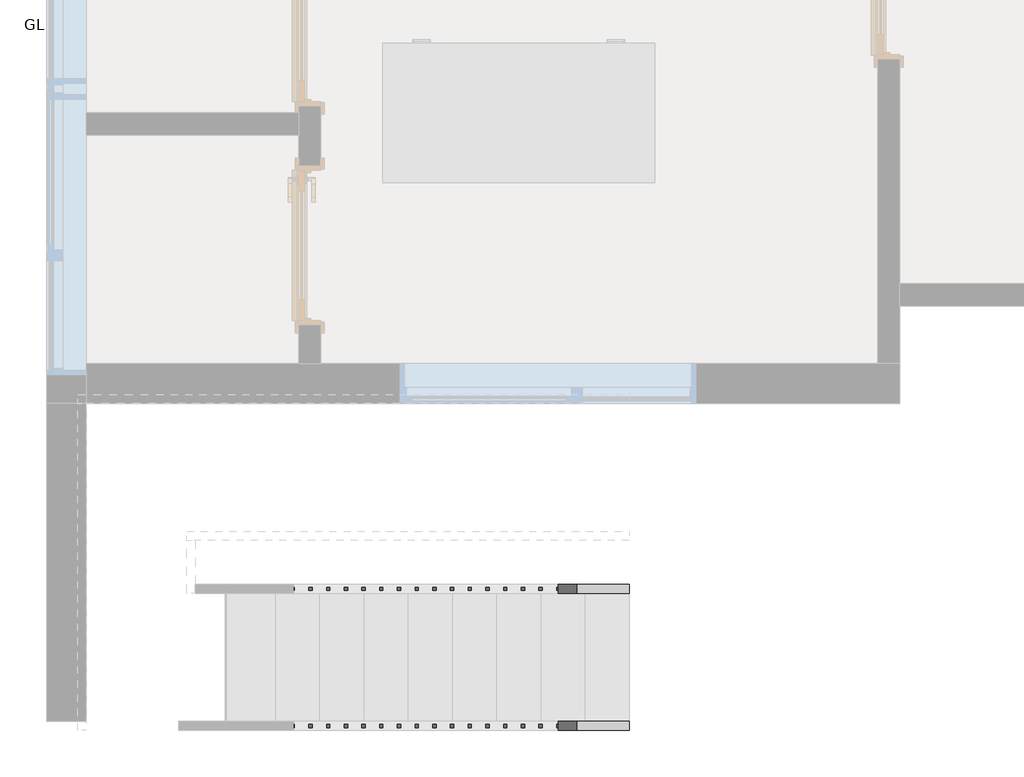
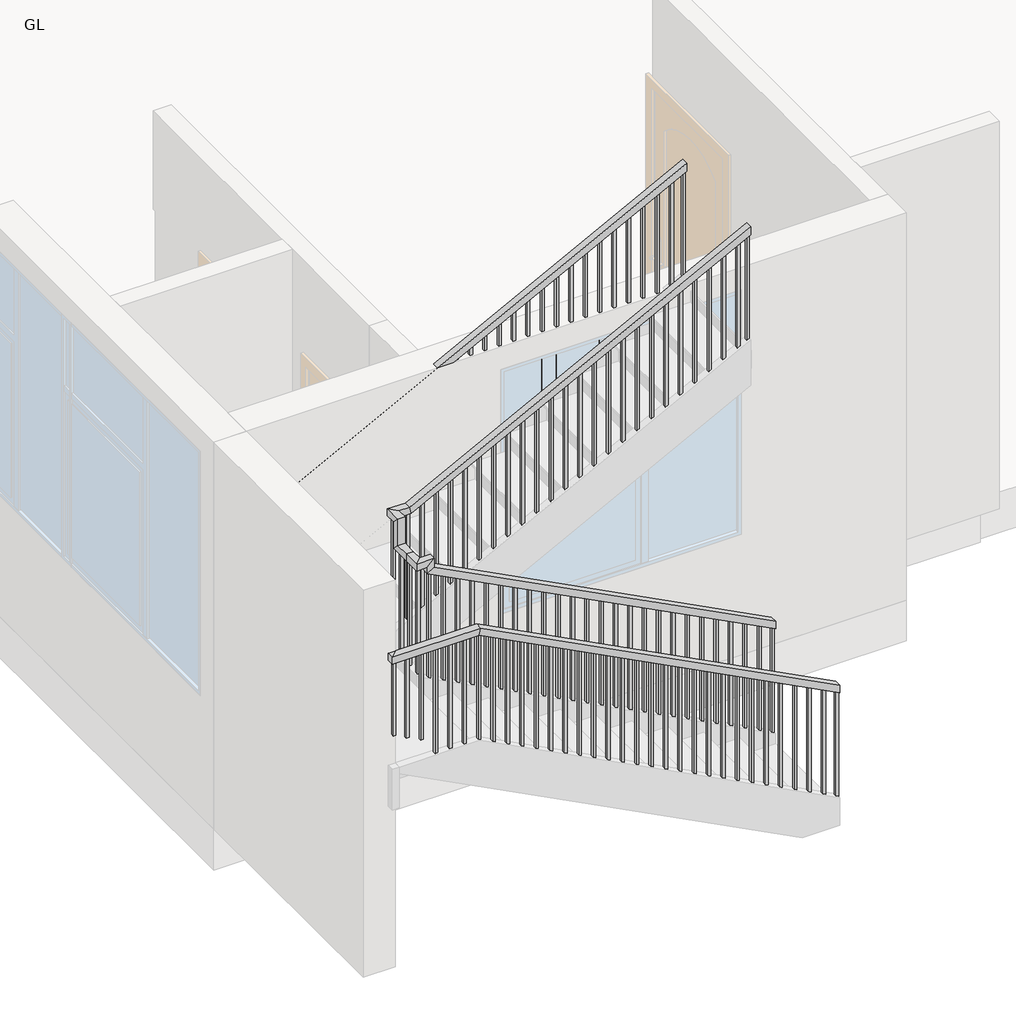
# One storey, part 3 of 4: 2 railings.
"""IFC4 building model written with IfcOpenShell, lengths in millimetres."""

from ifc_helpers import new_model, si_unit, frame, origin, place, context, project, spatial, polyline, outline, extrude, faceted_brep, element, save

model = new_model("IFC4")

# Units and contexts
model_context = context("Model", 3, world=origin())
ifc_project = project(units=[si_unit("LENGTHUNIT", "METRE", prefix="MILLI")], contexts=[model_context])

# Site, building, storey
site = spatial("IfcSite", under=ifc_project)
building = spatial("IfcBuilding", under=site)
storey = spatial("IfcBuildingStorey", under=building, Name="GL", Elevation=0.0)

# Railings
placement = place(None, origin())
element("IfcRailing", 1, ObjectType="Handrail - Rectangular", at=placement, inside=storey, context=model_context, shape_type="SolidModel", body=[
    faceted_brep([(-3117.2664982, -6914.3822004, 1046.0181818), (-3117.2664982, -6914.3822004, 988.803028), (-3117.2664982, -6863.5822004, 988.803028), (-3117.2664982, -6863.5822004, 1046.0181818), (-5530.2664982, -6914.3822004, 2296.3909091), (-5581.0664982, -6914.3822004, 2265.4993916), (-5581.0664982, -6863.5822004, 2265.4993916), (-5530.2664982, -6863.5822004, 2296.3909091), (-5657.2664982, -6787.3822004, 2311.4), (-5657.2664982, -6787.3822004, 2362.2), (-5657.2664982, -6685.7822004, 2362.2), (-5657.2664982, -6634.9822004, 2311.4), (-5606.4664982, -6787.3822004, 2311.4), (-5606.4664982, -6634.9822004, 2311.4), (-5606.4664982, -6787.3822004, 2362.2), (-5606.4664982, -6685.7822004, 2362.2), (-3117.2664982, -6558.7822004, 3810.0), (-3117.2664982, -6609.5822004, 3810.0), (-3117.2664982, -6609.5822004, 3752.7848461), (-3117.2664982, -6558.7822004, 3752.7848461), (-5517.8863767, -6558.7822004, 2508.8272727), (-5530.2664982, -6558.7822004, 2559.6272727), (-5517.8863767, -6609.5822004, 2508.8272727), (-5530.2664982, -6609.5822004, 2559.6272727), (-5530.2664982, -6914.3822004, 2362.2), (-5581.0664982, -6914.3822004, 2311.4), (-5581.0664982, -6863.5822004, 2311.4), (-5530.2664982, -6863.5822004, 2362.2), (-5657.2664982, -6914.3822004, 2362.2), (-5657.2664982, -6914.3822004, 2311.4), (-5606.4664982, -6863.5822004, 2311.4), (-5606.4664982, -6863.5822004, 2362.2), (-5657.2664982, -6685.7822004, 2559.6272727), (-5657.2664982, -6634.9822004, 2508.8272727), (-5606.4664982, -6634.9822004, 2508.8272727), (-5606.4664982, -6685.7822004, 2559.6272727), (-5657.2664982, -6558.7822004, 2559.6272727), (-5657.2664982, -6558.7822004, 2508.8272727), (-5606.4664982, -6609.5822004, 2508.8272727), (-5606.4664982, -6609.5822004, 2559.6272727)], [[[0, 1, 2, 3]], [[1, 0, 4, 5]], [[2, 1, 5, 6]], [[3, 2, 6, 7]], [[0, 3, 7, 4]], [[8, 9, 10, 11]], [[12, 8, 11, 13]], [[14, 12, 13, 15]], [[9, 14, 15, 10]], [[16, 17, 18, 19]], [[20, 21, 16, 19]], [[22, 20, 19, 18]], [[23, 22, 18, 17]], [[21, 23, 17, 16]], [[5, 4, 24, 25]], [[6, 5, 25, 26]], [[7, 6, 26, 27]], [[4, 7, 27, 24]], [[25, 24, 28, 29]], [[26, 25, 29, 30]], [[27, 26, 30, 31]], [[24, 27, 31, 28]], [[29, 28, 9, 8]], [[30, 29, 8, 12]], [[31, 30, 12, 14]], [[28, 31, 14, 9]], [[11, 10, 32, 33]], [[13, 11, 33, 34]], [[15, 13, 34, 35]], [[10, 15, 35, 32]], [[33, 32, 36, 37]], [[34, 33, 37, 38]], [[35, 34, 38, 39]], [[32, 35, 39, 36]], [[37, 36, 21, 20]], [[38, 37, 20, 22]], [[39, 38, 22, 23]], [[36, 39, 23, 21]]]),
    extrude(outline(polyline([(3718.2350734, -3183.9414982), (3708.3637098, -3202.9914982), (2924.0803899, -3202.9914982), (2933.9517536, -3183.9414982), (3718.2350734, -3183.9414982)])), frame((0.0, -6593.7072004, 0.0), z_axis=(0.0, 1.0, 0.0), x_axis=(0.0, 0.0, 1.0)), (0.0, 0.0, 1.0), 19.05),
    extrude(outline(polyline([(3665.5878007, -3285.5414982), (3655.716437, -3304.5914982), (2871.4331172, -3304.5914982), (2881.3044808, -3285.5414982), (3665.5878007, -3285.5414982)])), frame((0.0, -6593.7072004, 0.0), z_axis=(0.0, 1.0, 0.0), x_axis=(0.0, 0.0, 1.0)), (0.0, 0.0, 1.0), 19.05),
    extrude(outline(polyline([(3612.940528, -3387.1414982), (3603.0691643, -3406.1914982), (2818.7858445, -3406.1914982), (2828.6572081, -3387.1414982), (3612.940528, -3387.1414982)])), frame((0.0, -6593.7072004, 0.0), z_axis=(0.0, 1.0, 0.0), x_axis=(0.0, 0.0, 1.0)), (0.0, 0.0, 1.0), 19.05),
    extrude(outline(polyline([(3560.2932552, -3488.7414982), (3550.4218916, -3507.7914982), (2766.1385718, -3507.7914982), (2776.0099354, -3488.7414982), (3560.2932552, -3488.7414982)])), frame((0.0, -6593.7072004, 0.0), z_axis=(0.0, 1.0, 0.0), x_axis=(0.0, 0.0, 1.0)), (0.0, 0.0, 1.0), 19.05),
    extrude(outline(polyline([(3507.6459825, -3590.3414982), (3497.7746189, -3609.3914982), (2713.491299, -3609.3914982), (2723.3626627, -3590.3414982), (3507.6459825, -3590.3414982)])), frame((0.0, -6593.7072004, 0.0), z_axis=(0.0, 1.0, 0.0), x_axis=(0.0, 0.0, 1.0)), (0.0, 0.0, 1.0), 19.05),
    extrude(outline(polyline([(3454.9987098, -3691.9414982), (3445.1273461, -3710.9914982), (2660.8440263, -3710.9914982), (2670.7153899, -3691.9414982), (3454.9987098, -3691.9414982)])), frame((0.0, -6593.7072004, 0.0), z_axis=(0.0, 1.0, 0.0), x_axis=(0.0, 0.0, 1.0)), (0.0, 0.0, 1.0), 19.05),
    extrude(outline(polyline([(3402.351437, -3793.5414982), (3392.4800734, -3812.5914982), (2608.1967536, -3812.5914982), (2618.0681172, -3793.5414982), (3402.351437, -3793.5414982)])), frame((0.0, -6593.7072004, 0.0), z_axis=(0.0, 1.0, 0.0), x_axis=(0.0, 0.0, 1.0)), (0.0, 0.0, 1.0), 19.05),
    extrude(outline(polyline([(3349.7041643, -3895.1414982), (3339.8328007, -3914.1914982), (2555.5494808, -3914.1914982), (2565.4208445, -3895.1414982), (3349.7041643, -3895.1414982)])), frame((0.0, -6593.7072004, 0.0), z_axis=(0.0, 1.0, 0.0), x_axis=(0.0, 0.0, 1.0)), (0.0, 0.0, 1.0), 19.05),
    extrude(outline(polyline([(3297.0568916, -3996.7414982), (3287.185528, -4015.7914982), (2502.9022081, -4015.7914982), (2512.7735718, -3996.7414982), (3297.0568916, -3996.7414982)])), frame((0.0, -6593.7072004, 0.0), z_axis=(0.0, 1.0, 0.0), x_axis=(0.0, 0.0, 1.0)), (0.0, 0.0, 1.0), 19.05),
    extrude(outline(polyline([(3244.4096189, -4098.3414982), (3234.5382552, -4117.3914982), (2450.2549354, -4117.3914982), (2460.126299, -4098.3414982), (3244.4096189, -4098.3414982)])), frame((0.0, -6593.7072004, 0.0), z_axis=(0.0, 1.0, 0.0), x_axis=(0.0, 0.0, 1.0)), (0.0, 0.0, 1.0), 19.05),
    extrude(outline(polyline([(3191.7623461, -4199.9414982), (3181.8909825, -4218.9914982), (2397.6076627, -4218.9914982), (2407.4790263, -4199.9414982), (3191.7623461, -4199.9414982)])), frame((0.0, -6593.7072004, 0.0), z_axis=(0.0, 1.0, 0.0), x_axis=(0.0, 0.0, 1.0)), (0.0, 0.0, 1.0), 19.05),
    extrude(outline(polyline([(3139.1150734, -4301.5414982), (3129.2437098, -4320.5914982), (2344.9603899, -4320.5914982), (2354.8317536, -4301.5414982), (3139.1150734, -4301.5414982)])), frame((0.0, -6593.7072004, 0.0), z_axis=(0.0, 1.0, 0.0), x_axis=(0.0, 0.0, 1.0)), (0.0, 0.0, 1.0), 19.05),
    extrude(outline(polyline([(3086.4678007, -4403.1414982), (3076.596437, -4422.1914982), (2292.3131172, -4422.1914982), (2302.1844808, -4403.1414982), (3086.4678007, -4403.1414982)])), frame((0.0, -6593.7072004, 0.0), z_axis=(0.0, 1.0, 0.0), x_axis=(0.0, 0.0, 1.0)), (0.0, 0.0, 1.0), 19.05),
    extrude(outline(polyline([(3033.820528, -4504.7414982), (3023.9491643, -4523.7914982), (2239.6658445, -4523.7914982), (2249.5372081, -4504.7414982), (3033.820528, -4504.7414982)])), frame((0.0, -6593.7072004, 0.0), z_axis=(0.0, 1.0, 0.0), x_axis=(0.0, 0.0, 1.0)), (0.0, 0.0, 1.0), 19.05),
    extrude(outline(polyline([(2981.1732552, -4606.3414982), (2971.3018916, -4625.3914982), (2187.0185718, -4625.3914982), (2196.8899354, -4606.3414982), (2981.1732552, -4606.3414982)])), frame((0.0, -6593.7072004, 0.0), z_axis=(0.0, 1.0, 0.0), x_axis=(0.0, 0.0, 1.0)), (0.0, 0.0, 1.0), 19.05),
    extrude(outline(polyline([(2928.5259825, -4707.9414982), (2918.6546189, -4726.9914982), (2134.371299, -4726.9914982), (2144.2426627, -4707.9414982), (2928.5259825, -4707.9414982)])), frame((0.0, -6593.7072004, 0.0), z_axis=(0.0, 1.0, 0.0), x_axis=(0.0, 0.0, 1.0)), (0.0, 0.0, 1.0), 19.05),
    extrude(outline(polyline([(2875.8787098, -4809.5414982), (2866.0073461, -4828.5914982), (2081.7240263, -4828.5914982), (2091.5953899, -4809.5414982), (2875.8787098, -4809.5414982)])), frame((0.0, -6593.7072004, 0.0), z_axis=(0.0, 1.0, 0.0), x_axis=(0.0, 0.0, 1.0)), (0.0, 0.0, 1.0), 19.05),
    extrude(outline(polyline([(2823.231437, -4911.1414982), (2813.3600734, -4930.1914982), (2029.0767536, -4930.1914982), (2038.9481172, -4911.1414982), (2823.231437, -4911.1414982)])), frame((0.0, -6593.7072004, 0.0), z_axis=(0.0, 1.0, 0.0), x_axis=(0.0, 0.0, 1.0)), (0.0, 0.0, 1.0), 19.05),
    extrude(outline(polyline([(2770.5841643, -5012.7414982), (2760.7128007, -5031.7914982), (1976.4294808, -5031.7914982), (1986.3008445, -5012.7414982), (2770.5841643, -5012.7414982)])), frame((0.0, -6593.7072004, 0.0), z_axis=(0.0, 1.0, 0.0), x_axis=(0.0, 0.0, 1.0)), (0.0, 0.0, 1.0), 19.05),
    extrude(outline(polyline([(2717.9368916, -5114.3414982), (2708.065528, -5133.3914982), (1923.7822081, -5133.3914982), (1933.6535718, -5114.3414982), (2717.9368916, -5114.3414982)])), frame((0.0, -6593.7072004, 0.0), z_axis=(0.0, 1.0, 0.0), x_axis=(0.0, 0.0, 1.0)), (0.0, 0.0, 1.0), 19.05),
    extrude(outline(polyline([(2665.2896189, -5215.9414982), (2655.4182552, -5234.9914982), (1871.1349354, -5234.9914982), (1881.006299, -5215.9414982), (2665.2896189, -5215.9414982)])), frame((0.0, -6593.7072004, 0.0), z_axis=(0.0, 1.0, 0.0), x_axis=(0.0, 0.0, 1.0)), (0.0, 0.0, 1.0), 19.05),
    extrude(outline(polyline([(2612.6423461, -5317.5414982), (2602.7709825, -5336.5914982), (1818.4876627, -5336.5914982), (1828.3590263, -5317.5414982), (2612.6423461, -5317.5414982)])), frame((0.0, -6593.7072004, 0.0), z_axis=(0.0, 1.0, 0.0), x_axis=(0.0, 0.0, 1.0)), (0.0, 0.0, 1.0), 19.05),
    extrude(outline(polyline([(2559.9950734, -5419.1414982), (2550.1237098, -5438.1914982), (1765.8403899, -5438.1914982), (1775.7117536, -5419.1414982), (2559.9950734, -5419.1414982)])), frame((0.0, -6593.7072004, 0.0), z_axis=(0.0, 1.0, 0.0), x_axis=(0.0, 0.0, 1.0)), (0.0, 0.0, 1.0), 19.05),
    extrude(outline(polyline([(2507.3478007, -5520.7414982), (2497.476437, -5539.7914982), (1713.1931172, -5539.7914982), (1723.0644808, -5520.7414982), (2507.3478007, -5520.7414982)])), frame((0.0, -6593.7072004, 0.0), z_axis=(0.0, 1.0, 0.0), x_axis=(0.0, 0.0, 1.0)), (0.0, 0.0, 1.0), 19.05),
    extrude(outline(polyline([(-5622.3414982, -6695.3072004), (-5641.3914982, -6695.3072004), (-5641.3914982, -6676.2572004), (-5622.3414982, -6676.2572004), (-5622.3414982, -6695.3072004)])), frame((0.0, 0.0, 1524.0), z_axis=(0.0, 0.0, 1.0), x_axis=(1.0, 0.0, 0.0)), (0.0, 0.0, 1.0), 787.4),
    extrude(outline(polyline([(-5622.3414982, -6796.9072004), (-5641.3914982, -6796.9072004), (-5641.3914982, -6777.8572004), (-5622.3414982, -6777.8572004), (-5622.3414982, -6796.9072004)])), frame((0.0, 0.0, 1524.0), z_axis=(0.0, 0.0, 1.0), x_axis=(1.0, 0.0, 0.0)), (0.0, 0.0, 1.0), 787.4),
    extrude(outline(polyline([(2311.4, -5546.1414982), (2311.4, -5565.1914982), (1472.9899354, -5565.1914982), (1463.1185718, -5546.1414982), (2311.4, -5546.1414982)])), frame((0.0, -6898.5072004, 0.0), z_axis=(0.0, 1.0, 0.0), x_axis=(0.0, 0.0, 1.0)), (0.0, 0.0, 1.0), 19.05),
    extrude(outline(polyline([(2194.7546189, -5444.5414982), (2204.6259825, -5463.5914982), (1420.3426627, -5463.5914982), (1410.471299, -5444.5414982), (2194.7546189, -5444.5414982)])), frame((0.0, -6898.5072004, 0.0), z_axis=(0.0, 1.0, 0.0), x_axis=(0.0, 0.0, 1.0)), (0.0, 0.0, 1.0), 19.05),
    extrude(outline(polyline([(2142.1073461, -5342.9414982), (2151.9787098, -5361.9914982), (1367.6953899, -5361.9914982), (1357.8240263, -5342.9414982), (2142.1073461, -5342.9414982)])), frame((0.0, -6898.5072004, 0.0), z_axis=(0.0, 1.0, 0.0), x_axis=(0.0, 0.0, 1.0)), (0.0, 0.0, 1.0), 19.05),
    extrude(outline(polyline([(2089.4600734, -5241.3414982), (2099.331437, -5260.3914982), (1315.0481172, -5260.3914982), (1305.1767536, -5241.3414982), (2089.4600734, -5241.3414982)])), frame((0.0, -6898.5072004, 0.0), z_axis=(0.0, 1.0, 0.0), x_axis=(0.0, 0.0, 1.0)), (0.0, 0.0, 1.0), 19.05),
    extrude(outline(polyline([(2036.8128007, -5139.7414982), (2046.6841643, -5158.7914982), (1262.4008445, -5158.7914982), (1252.5294808, -5139.7414982), (2036.8128007, -5139.7414982)])), frame((0.0, -6898.5072004, 0.0), z_axis=(0.0, 1.0, 0.0), x_axis=(0.0, 0.0, 1.0)), (0.0, 0.0, 1.0), 19.05),
    extrude(outline(polyline([(1984.165528, -5038.1414982), (1994.0368916, -5057.1914982), (1209.7535718, -5057.1914982), (1199.8822081, -5038.1414982), (1984.165528, -5038.1414982)])), frame((0.0, -6898.5072004, 0.0), z_axis=(0.0, 1.0, 0.0), x_axis=(0.0, 0.0, 1.0)), (0.0, 0.0, 1.0), 19.05),
    extrude(outline(polyline([(1931.5182552, -4936.5414982), (1941.3896189, -4955.5914982), (1157.106299, -4955.5914982), (1147.2349354, -4936.5414982), (1931.5182552, -4936.5414982)])), frame((0.0, -6898.5072004, 0.0), z_axis=(0.0, 1.0, 0.0), x_axis=(0.0, 0.0, 1.0)), (0.0, 0.0, 1.0), 19.05),
    extrude(outline(polyline([(1878.8709825, -4834.9414982), (1888.7423461, -4853.9914982), (1104.4590263, -4853.9914982), (1094.5876627, -4834.9414982), (1878.8709825, -4834.9414982)])), frame((0.0, -6898.5072004, 0.0), z_axis=(0.0, 1.0, 0.0), x_axis=(0.0, 0.0, 1.0)), (0.0, 0.0, 1.0), 19.05),
    extrude(outline(polyline([(1826.2237098, -4733.3414982), (1836.0950734, -4752.3914982), (1051.8117536, -4752.3914982), (1041.9403899, -4733.3414982), (1826.2237098, -4733.3414982)])), frame((0.0, -6898.5072004, 0.0), z_axis=(0.0, 1.0, 0.0), x_axis=(0.0, 0.0, 1.0)), (0.0, 0.0, 1.0), 19.05),
    extrude(outline(polyline([(1773.576437, -4631.7414982), (1783.4478007, -4650.7914982), (999.1644808, -4650.7914982), (989.2931172, -4631.7414982), (1773.576437, -4631.7414982)])), frame((0.0, -6898.5072004, 0.0), z_axis=(0.0, 1.0, 0.0), x_axis=(0.0, 0.0, 1.0)), (0.0, 0.0, 1.0), 19.05),
    extrude(outline(polyline([(1720.9291643, -4530.1414982), (1730.800528, -4549.1914982), (946.5172081, -4549.1914982), (936.6458445, -4530.1414982), (1720.9291643, -4530.1414982)])), frame((0.0, -6898.5072004, 0.0), z_axis=(0.0, 1.0, 0.0), x_axis=(0.0, 0.0, 1.0)), (0.0, 0.0, 1.0), 19.05),
    extrude(outline(polyline([(1668.2818916, -4428.5414982), (1678.1532552, -4447.5914982), (893.8699354, -4447.5914982), (883.9985718, -4428.5414982), (1668.2818916, -4428.5414982)])), frame((0.0, -6898.5072004, 0.0), z_axis=(0.0, 1.0, 0.0), x_axis=(0.0, 0.0, 1.0)), (0.0, 0.0, 1.0), 19.05),
    extrude(outline(polyline([(1615.6346189, -4326.9414982), (1625.5059825, -4345.9914982), (841.2226627, -4345.9914982), (831.351299, -4326.9414982), (1615.6346189, -4326.9414982)])), frame((0.0, -6898.5072004, 0.0), z_axis=(0.0, 1.0, 0.0), x_axis=(0.0, 0.0, 1.0)), (0.0, 0.0, 1.0), 19.05),
    extrude(outline(polyline([(1562.9873461, -4225.3414982), (1572.8587098, -4244.3914982), (788.5753899, -4244.3914982), (778.7040263, -4225.3414982), (1562.9873461, -4225.3414982)])), frame((0.0, -6898.5072004, 0.0), z_axis=(0.0, 1.0, 0.0), x_axis=(0.0, 0.0, 1.0)), (0.0, 0.0, 1.0), 19.05),
    extrude(outline(polyline([(1510.3400734, -4123.7414982), (1520.211437, -4142.7914982), (735.9281172, -4142.7914982), (726.0567536, -4123.7414982), (1510.3400734, -4123.7414982)])), frame((0.0, -6898.5072004, 0.0), z_axis=(0.0, 1.0, 0.0), x_axis=(0.0, 0.0, 1.0)), (0.0, 0.0, 1.0), 19.05),
    extrude(outline(polyline([(1457.6928007, -4022.1414982), (1467.5641643, -4041.1914982), (683.2808445, -4041.1914982), (673.4094808, -4022.1414982), (1457.6928007, -4022.1414982)])), frame((0.0, -6898.5072004, 0.0), z_axis=(0.0, 1.0, 0.0), x_axis=(0.0, 0.0, 1.0)), (0.0, 0.0, 1.0), 19.05),
    extrude(outline(polyline([(1405.045528, -3920.5414982), (1414.9168916, -3939.5914982), (630.6335718, -3939.5914982), (620.7622081, -3920.5414982), (1405.045528, -3920.5414982)])), frame((0.0, -6898.5072004, 0.0), z_axis=(0.0, 1.0, 0.0), x_axis=(0.0, 0.0, 1.0)), (0.0, 0.0, 1.0), 19.05),
    extrude(outline(polyline([(1352.3982552, -3818.9414982), (1362.2696189, -3837.9914982), (577.986299, -3837.9914982), (568.1149354, -3818.9414982), (1352.3982552, -3818.9414982)])), frame((0.0, -6898.5072004, 0.0), z_axis=(0.0, 1.0, 0.0), x_axis=(0.0, 0.0, 1.0)), (0.0, 0.0, 1.0), 19.05),
    extrude(outline(polyline([(1299.7509825, -3717.3414982), (1309.6223461, -3736.3914982), (525.3390263, -3736.3914982), (515.4676627, -3717.3414982), (1299.7509825, -3717.3414982)])), frame((0.0, -6898.5072004, 0.0), z_axis=(0.0, 1.0, 0.0), x_axis=(0.0, 0.0, 1.0)), (0.0, 0.0, 1.0), 19.05),
    extrude(outline(polyline([(1247.1037098, -3615.7414982), (1256.9750734, -3634.7914982), (472.6917536, -3634.7914982), (462.8203899, -3615.7414982), (1247.1037098, -3615.7414982)])), frame((0.0, -6898.5072004, 0.0), z_axis=(0.0, 1.0, 0.0), x_axis=(0.0, 0.0, 1.0)), (0.0, 0.0, 1.0), 19.05),
    extrude(outline(polyline([(1194.456437, -3514.1414982), (1204.3278007, -3533.1914982), (420.0444808, -3533.1914982), (410.1731172, -3514.1414982), (1194.456437, -3514.1414982)])), frame((0.0, -6898.5072004, 0.0), z_axis=(0.0, 1.0, 0.0), x_axis=(0.0, 0.0, 1.0)), (0.0, 0.0, 1.0), 19.05),
    extrude(outline(polyline([(1141.8091643, -3412.5414982), (1151.680528, -3431.5914982), (367.3972081, -3431.5914982), (357.5258445, -3412.5414982), (1141.8091643, -3412.5414982)])), frame((0.0, -6898.5072004, 0.0), z_axis=(0.0, 1.0, 0.0), x_axis=(0.0, 0.0, 1.0)), (0.0, 0.0, 1.0), 19.05),
    extrude(outline(polyline([(1089.1618916, -3310.9414982), (1099.0332552, -3329.9914982), (314.7499354, -3329.9914982), (304.8785718, -3310.9414982), (1089.1618916, -3310.9414982)])), frame((0.0, -6898.5072004, 0.0), z_axis=(0.0, 1.0, 0.0), x_axis=(0.0, 0.0, 1.0)), (0.0, 0.0, 1.0), 19.05),
    extrude(outline(polyline([(1036.5146189, -3209.3414982), (1046.3859825, -3228.3914982), (262.1026627, -3228.3914982), (252.231299, -3209.3414982), (1036.5146189, -3209.3414982)])), frame((0.0, -6898.5072004, 0.0), z_axis=(0.0, 1.0, 0.0), x_axis=(0.0, 0.0, 1.0)), (0.0, 0.0, 1.0), 19.05),
    extrude(outline(polyline([(-6593.7072004, 2508.8272727), (-6574.6572004, 2508.8272727), (-6574.6572004, 1670.4172081), (-6593.7072004, 1660.5458445), (-6593.7072004, 2508.8272727)])), frame((-5641.3914982, 0.0, 0.0), z_axis=(1.0, 0.0, 0.0), x_axis=(0.0, 1.0, 0.0)), (0.0, 0.0, 1.0), 19.05),
    extrude(outline(polyline([(-5622.3414982, -6879.4572004), (-5622.3414982, -6898.5072004), (-5641.3914982, -6898.5072004), (-5641.3914982, -6879.4572004), (-5622.3414982, -6879.4572004)])), frame((0.0, 0.0, 1524.0), z_axis=(0.0, 0.0, 1.0), x_axis=(1.0, 0.0, 0.0)), (0.0, 0.0, 1.0), 787.4),
    extrude(outline(polyline([(3752.7848461, -3117.2664982), (3742.9134825, -3136.3164982), (2958.6301627, -3136.3164982), (2968.5015263, -3117.2664982), (3752.7848461, -3117.2664982)])), frame((0.0, -6593.7072004, 0.0), z_axis=(0.0, 1.0, 0.0), x_axis=(0.0, 0.0, 1.0)), (0.0, 0.0, 1.0), 19.05),
    extrude(outline(polyline([(988.803028, -3117.2664982), (998.6743916, -3136.3164982), (214.3910718, -3136.3164982), (204.5197081, -3117.2664982), (988.803028, -3117.2664982)])), frame((0.0, -6898.5072004, 0.0), z_axis=(0.0, 1.0, 0.0), x_axis=(0.0, 0.0, 1.0)), (0.0, 0.0, 1.0), 19.05),
])
element("IfcRailing", 2, ObjectType="Handrail - Rectangular", at=placement, inside=storey, context=model_context, shape_type="SolidModel", body=[
    faceted_brep([(-3117.2664982, -7701.7822004, 1046.0181818), (-3117.2664982, -7701.7822004, 988.803028), (-3117.2664982, -7650.9822004, 988.803028), (-3117.2664982, -7650.9822004, 1046.0181818), (-5657.2664982, -7701.7822004, 2362.2), (-5669.6466197, -7701.7822004, 2311.4), (-5669.6466197, -7650.9822004, 2311.4), (-5657.2664982, -7650.9822004, 2362.2), (-6283.3131972, -7701.7822004, 2311.4), (-6283.3131972, -7701.7822004, 2362.2), (-6283.3131972, -5773.9082131, 2362.2), (-6283.3131972, -5773.9082131, 2311.4), (-6232.5131972, -7650.9822004, 2311.4), (-6232.5131972, -5824.7082131, 2311.4), (-6232.5131972, -7650.9822004, 2362.2), (-6232.5131972, -5824.7082131, 2362.2), (-5911.2664982, -5773.9082131, 2362.2), (-5898.8863767, -5773.9082131, 2311.4), (-5898.8863767, -5824.7082131, 2311.4), (-5911.2664982, -5824.7082131, 2362.2), (-3117.2664982, -5773.9082131, 3810.0), (-3117.2664982, -5824.7082131, 3810.0), (-3117.2664982, -5824.7082131, 3752.7848461), (-3117.2664982, -5773.9082131, 3752.7848461)], [[[0, 1, 2, 3]], [[1, 0, 4, 5]], [[2, 1, 5, 6]], [[3, 2, 6, 7]], [[0, 3, 7, 4]], [[8, 9, 10, 11]], [[12, 8, 11, 13]], [[14, 12, 13, 15]], [[9, 14, 15, 10]], [[11, 10, 16, 17]], [[13, 11, 17, 18]], [[15, 13, 18, 19]], [[10, 15, 19, 16]], [[5, 4, 9, 8]], [[6, 5, 8, 12]], [[7, 6, 12, 14]], [[4, 7, 14, 9]], [[20, 21, 22, 23]], [[17, 16, 20, 23]], [[18, 17, 23, 22]], [[19, 18, 22, 21]], [[16, 19, 21, 20]]]),
    extrude(outline(polyline([(3699.8413294, -3219.4381972), (2915.5580095, -3219.4381972), (2925.4293732, -3200.3881972), (3709.712693, -3200.3881972), (3699.8413294, -3219.4381972)])), frame((0.0, -5808.8332131, 0.0), z_axis=(0.0, 1.0, 0.0), x_axis=(0.0, 0.0, 1.0)), (0.0, 0.0, 1.0), 19.05),
    extrude(outline(polyline([(3647.1940566, -3321.0381972), (2862.9107368, -3321.0381972), (2872.7821004, -3301.9881972), (3657.0654203, -3301.9881972), (3647.1940566, -3321.0381972)])), frame((0.0, -5808.8332131, 0.0), z_axis=(0.0, 1.0, 0.0), x_axis=(0.0, 0.0, 1.0)), (0.0, 0.0, 1.0), 19.05),
    extrude(outline(polyline([(3594.5467839, -3422.6381972), (2810.2634641, -3422.6381972), (2820.1348277, -3403.5881972), (3604.4181476, -3403.5881972), (3594.5467839, -3422.6381972)])), frame((0.0, -5808.8332131, 0.0), z_axis=(0.0, 1.0, 0.0), x_axis=(0.0, 0.0, 1.0)), (0.0, 0.0, 1.0), 19.05),
    extrude(outline(polyline([(3541.8995112, -3524.2381972), (2757.6161913, -3524.2381972), (2767.487555, -3505.1881972), (3551.7708748, -3505.1881972), (3541.8995112, -3524.2381972)])), frame((0.0, -5808.8332131, 0.0), z_axis=(0.0, 1.0, 0.0), x_axis=(0.0, 0.0, 1.0)), (0.0, 0.0, 1.0), 19.05),
    extrude(outline(polyline([(3489.2522385, -3625.8381972), (2704.9689186, -3625.8381972), (2714.8402823, -3606.7881972), (3499.1236021, -3606.7881972), (3489.2522385, -3625.8381972)])), frame((0.0, -5808.8332131, 0.0), z_axis=(0.0, 1.0, 0.0), x_axis=(0.0, 0.0, 1.0)), (0.0, 0.0, 1.0), 19.05),
    extrude(outline(polyline([(3436.6049657, -3727.4381972), (2652.3216459, -3727.4381972), (2662.1930095, -3708.3881972), (3446.4763294, -3708.3881972), (3436.6049657, -3727.4381972)])), frame((0.0, -5808.8332131, 0.0), z_axis=(0.0, 1.0, 0.0), x_axis=(0.0, 0.0, 1.0)), (0.0, 0.0, 1.0), 19.05),
    extrude(outline(polyline([(3383.957693, -3829.0381972), (2599.6743732, -3829.0381972), (2609.5457368, -3809.9881972), (3393.8290566, -3809.9881972), (3383.957693, -3829.0381972)])), frame((0.0, -5808.8332131, 0.0), z_axis=(0.0, 1.0, 0.0), x_axis=(0.0, 0.0, 1.0)), (0.0, 0.0, 1.0), 19.05),
    extrude(outline(polyline([(3331.3104203, -3930.6381972), (2547.0271004, -3930.6381972), (2556.8984641, -3911.5881972), (3341.1817839, -3911.5881972), (3331.3104203, -3930.6381972)])), frame((0.0, -5808.8332131, 0.0), z_axis=(0.0, 1.0, 0.0), x_axis=(0.0, 0.0, 1.0)), (0.0, 0.0, 1.0), 19.05),
    extrude(outline(polyline([(3278.6631476, -4032.2381972), (2494.3798277, -4032.2381972), (2504.2511913, -4013.1881972), (3288.5345112, -4013.1881972), (3278.6631476, -4032.2381972)])), frame((0.0, -5808.8332131, 0.0), z_axis=(0.0, 1.0, 0.0), x_axis=(0.0, 0.0, 1.0)), (0.0, 0.0, 1.0), 19.05),
    extrude(outline(polyline([(3226.0158748, -4133.8381972), (2441.732555, -4133.8381972), (2451.6039186, -4114.7881972), (3235.8872385, -4114.7881972), (3226.0158748, -4133.8381972)])), frame((0.0, -5808.8332131, 0.0), z_axis=(0.0, 1.0, 0.0), x_axis=(0.0, 0.0, 1.0)), (0.0, 0.0, 1.0), 19.05),
    extrude(outline(polyline([(3173.3686021, -4235.4381972), (2389.0852823, -4235.4381972), (2398.9566459, -4216.3881972), (3183.2399657, -4216.3881972), (3173.3686021, -4235.4381972)])), frame((0.0, -5808.8332131, 0.0), z_axis=(0.0, 1.0, 0.0), x_axis=(0.0, 0.0, 1.0)), (0.0, 0.0, 1.0), 19.05),
    extrude(outline(polyline([(3120.7213294, -4337.0381972), (2336.4380095, -4337.0381972), (2346.3093732, -4317.9881972), (3130.592693, -4317.9881972), (3120.7213294, -4337.0381972)])), frame((0.0, -5808.8332131, 0.0), z_axis=(0.0, 1.0, 0.0), x_axis=(0.0, 0.0, 1.0)), (0.0, 0.0, 1.0), 19.05),
    extrude(outline(polyline([(3068.0740566, -4438.6381972), (2283.7907368, -4438.6381972), (2293.6621004, -4419.5881972), (3077.9454203, -4419.5881972), (3068.0740566, -4438.6381972)])), frame((0.0, -5808.8332131, 0.0), z_axis=(0.0, 1.0, 0.0), x_axis=(0.0, 0.0, 1.0)), (0.0, 0.0, 1.0), 19.05),
    extrude(outline(polyline([(3015.4267839, -4540.2381972), (2231.1434641, -4540.2381972), (2241.0148277, -4521.1881972), (3025.2981476, -4521.1881972), (3015.4267839, -4540.2381972)])), frame((0.0, -5808.8332131, 0.0), z_axis=(0.0, 1.0, 0.0), x_axis=(0.0, 0.0, 1.0)), (0.0, 0.0, 1.0), 19.05),
    extrude(outline(polyline([(2962.7795112, -4641.8381972), (2178.4961913, -4641.8381972), (2188.367555, -4622.7881972), (2972.6508748, -4622.7881972), (2962.7795112, -4641.8381972)])), frame((0.0, -5808.8332131, 0.0), z_axis=(0.0, 1.0, 0.0), x_axis=(0.0, 0.0, 1.0)), (0.0, 0.0, 1.0), 19.05),
    extrude(outline(polyline([(2910.1322385, -4743.4381972), (2125.8489186, -4743.4381972), (2135.7202823, -4724.3881972), (2920.0036021, -4724.3881972), (2910.1322385, -4743.4381972)])), frame((0.0, -5808.8332131, 0.0), z_axis=(0.0, 1.0, 0.0), x_axis=(0.0, 0.0, 1.0)), (0.0, 0.0, 1.0), 19.05),
    extrude(outline(polyline([(2857.4849657, -4845.0381972), (2073.2016459, -4845.0381972), (2083.0730095, -4825.9881972), (2867.3563294, -4825.9881972), (2857.4849657, -4845.0381972)])), frame((0.0, -5808.8332131, 0.0), z_axis=(0.0, 1.0, 0.0), x_axis=(0.0, 0.0, 1.0)), (0.0, 0.0, 1.0), 19.05),
    extrude(outline(polyline([(2804.837693, -4946.6381972), (2020.5543732, -4946.6381972), (2030.4257368, -4927.5881972), (2814.7090566, -4927.5881972), (2804.837693, -4946.6381972)])), frame((0.0, -5808.8332131, 0.0), z_axis=(0.0, 1.0, 0.0), x_axis=(0.0, 0.0, 1.0)), (0.0, 0.0, 1.0), 19.05),
    extrude(outline(polyline([(2752.1904203, -5048.2381972), (1967.9071004, -5048.2381972), (1977.7784641, -5029.1881972), (2762.0617839, -5029.1881972), (2752.1904203, -5048.2381972)])), frame((0.0, -5808.8332131, 0.0), z_axis=(0.0, 1.0, 0.0), x_axis=(0.0, 0.0, 1.0)), (0.0, 0.0, 1.0), 19.05),
    extrude(outline(polyline([(2699.5431476, -5149.8381972), (1915.2598277, -5149.8381972), (1925.1311913, -5130.7881972), (2709.4145112, -5130.7881972), (2699.5431476, -5149.8381972)])), frame((0.0, -5808.8332131, 0.0), z_axis=(0.0, 1.0, 0.0), x_axis=(0.0, 0.0, 1.0)), (0.0, 0.0, 1.0), 19.05),
    extrude(outline(polyline([(2646.8958748, -5251.4381972), (1862.612555, -5251.4381972), (1872.4839186, -5232.3881972), (2656.7672385, -5232.3881972), (2646.8958748, -5251.4381972)])), frame((0.0, -5808.8332131, 0.0), z_axis=(0.0, 1.0, 0.0), x_axis=(0.0, 0.0, 1.0)), (0.0, 0.0, 1.0), 19.05),
    extrude(outline(polyline([(2594.2486021, -5353.0381972), (1809.9652823, -5353.0381972), (1819.8366459, -5333.9881972), (2604.1199657, -5333.9881972), (2594.2486021, -5353.0381972)])), frame((0.0, -5808.8332131, 0.0), z_axis=(0.0, 1.0, 0.0), x_axis=(0.0, 0.0, 1.0)), (0.0, 0.0, 1.0), 19.05),
    extrude(outline(polyline([(2541.6013294, -5454.6381972), (1757.3180095, -5454.6381972), (1767.1893732, -5435.5881972), (2551.472693, -5435.5881972), (2541.6013294, -5454.6381972)])), frame((0.0, -5808.8332131, 0.0), z_axis=(0.0, 1.0, 0.0), x_axis=(0.0, 0.0, 1.0)), (0.0, 0.0, 1.0), 19.05),
    extrude(outline(polyline([(2488.9540566, -5556.2381972), (1704.6707368, -5556.2381972), (1714.5421004, -5537.1881972), (2498.8254203, -5537.1881972), (2488.9540566, -5556.2381972)])), frame((0.0, -5808.8332131, 0.0), z_axis=(0.0, 1.0, 0.0), x_axis=(0.0, 0.0, 1.0)), (0.0, 0.0, 1.0), 19.05),
    extrude(outline(polyline([(2436.3067839, -5657.8381972), (1652.0234641, -5657.8381972), (1661.8948277, -5638.7881972), (2446.1781476, -5638.7881972), (2436.3067839, -5657.8381972)])), frame((0.0, -5808.8332131, 0.0), z_axis=(0.0, 1.0, 0.0), x_axis=(0.0, 0.0, 1.0)), (0.0, 0.0, 1.0), 19.05),
    extrude(outline(polyline([(2383.6595112, -5759.4381972), (1599.3761913, -5759.4381972), (1609.247555, -5740.3881972), (2393.5308748, -5740.3881972), (2383.6595112, -5759.4381972)])), frame((0.0, -5808.8332131, 0.0), z_axis=(0.0, 1.0, 0.0), x_axis=(0.0, 0.0, 1.0)), (0.0, 0.0, 1.0), 19.05),
    extrude(outline(polyline([(2331.0122385, -5861.0381972), (1546.7289186, -5861.0381972), (1556.6002823, -5841.9881972), (2340.8836021, -5841.9881972), (2331.0122385, -5861.0381972)])), frame((0.0, -5808.8332131, 0.0), z_axis=(0.0, 1.0, 0.0), x_axis=(0.0, 0.0, 1.0)), (0.0, 0.0, 1.0), 19.05),
    extrude(outline(polyline([(2311.4, -5962.6381972), (1494.0816459, -5962.6381972), (1503.9530095, -5943.5881972), (2311.4, -5943.5881972), (2311.4, -5962.6381972)])), frame((0.0, -5808.8332131, 0.0), z_axis=(0.0, 1.0, 0.0), x_axis=(0.0, 0.0, 1.0)), (0.0, 0.0, 1.0), 19.05),
    extrude(outline(polyline([(2311.4, -6064.2381972), (1441.4343732, -6064.2381972), (1451.3057368, -6045.1881972), (2311.4, -6045.1881972), (2311.4, -6064.2381972)])), frame((0.0, -5808.8332131, 0.0), z_axis=(0.0, 1.0, 0.0), x_axis=(0.0, 0.0, 1.0)), (0.0, 0.0, 1.0), 19.05),
    extrude(outline(polyline([(2311.4, -6165.8381972), (1388.7871004, -6165.8381972), (1398.6584641, -6146.7881972), (2311.4, -6146.7881972), (2311.4, -6165.8381972)])), frame((0.0, -5808.8332131, 0.0), z_axis=(0.0, 1.0, 0.0), x_axis=(0.0, 0.0, 1.0)), (0.0, 0.0, 1.0), 19.05),
    extrude(outline(polyline([(-6267.4381972, -5857.1072004), (-6267.4381972, -5838.0572004), (-6248.3881972, -5838.0572004), (-6248.3881972, -5857.1072004), (-6267.4381972, -5857.1072004)])), frame((0.0, 0.0, 1524.0), z_axis=(0.0, 0.0, 1.0), x_axis=(1.0, 0.0, 0.0)), (0.0, 0.0, 1.0), 787.4),
    extrude(outline(polyline([(-6267.4381972, -5958.7072004), (-6267.4381972, -5939.6572004), (-6248.3881972, -5939.6572004), (-6248.3881972, -5958.7072004), (-6267.4381972, -5958.7072004)])), frame((0.0, 0.0, 1524.0), z_axis=(0.0, 0.0, 1.0), x_axis=(1.0, 0.0, 0.0)), (0.0, 0.0, 1.0), 787.4),
    extrude(outline(polyline([(-6267.4381972, -6060.3072004), (-6267.4381972, -6041.2572004), (-6248.3881972, -6041.2572004), (-6248.3881972, -6060.3072004), (-6267.4381972, -6060.3072004)])), frame((0.0, 0.0, 1524.0), z_axis=(0.0, 0.0, 1.0), x_axis=(1.0, 0.0, 0.0)), (0.0, 0.0, 1.0), 787.4),
    extrude(outline(polyline([(-6267.4381972, -6161.9072004), (-6267.4381972, -6142.8572004), (-6248.3881972, -6142.8572004), (-6248.3881972, -6161.9072004), (-6267.4381972, -6161.9072004)])), frame((0.0, 0.0, 1524.0), z_axis=(0.0, 0.0, 1.0), x_axis=(1.0, 0.0, 0.0)), (0.0, 0.0, 1.0), 787.4),
    extrude(outline(polyline([(-6267.4381972, -6263.5072004), (-6267.4381972, -6244.4572004), (-6248.3881972, -6244.4572004), (-6248.3881972, -6263.5072004), (-6267.4381972, -6263.5072004)])), frame((0.0, 0.0, 1524.0), z_axis=(0.0, 0.0, 1.0), x_axis=(1.0, 0.0, 0.0)), (0.0, 0.0, 1.0), 787.4),
    extrude(outline(polyline([(-6267.4381972, -6365.1072004), (-6267.4381972, -6346.0572004), (-6248.3881972, -6346.0572004), (-6248.3881972, -6365.1072004), (-6267.4381972, -6365.1072004)])), frame((0.0, 0.0, 1524.0), z_axis=(0.0, 0.0, 1.0), x_axis=(1.0, 0.0, 0.0)), (0.0, 0.0, 1.0), 787.4),
    extrude(outline(polyline([(-6267.4381972, -6466.7072004), (-6267.4381972, -6447.6572004), (-6248.3881972, -6447.6572004), (-6248.3881972, -6466.7072004), (-6267.4381972, -6466.7072004)])), frame((0.0, 0.0, 1524.0), z_axis=(0.0, 0.0, 1.0), x_axis=(1.0, 0.0, 0.0)), (0.0, 0.0, 1.0), 787.4),
    extrude(outline(polyline([(-6267.4381972, -6568.3072004), (-6267.4381972, -6549.2572004), (-6248.3881972, -6549.2572004), (-6248.3881972, -6568.3072004), (-6267.4381972, -6568.3072004)])), frame((0.0, 0.0, 1524.0), z_axis=(0.0, 0.0, 1.0), x_axis=(1.0, 0.0, 0.0)), (0.0, 0.0, 1.0), 787.4),
    extrude(outline(polyline([(-6267.4381972, -6669.9072004), (-6267.4381972, -6650.8572004), (-6248.3881972, -6650.8572004), (-6248.3881972, -6669.9072004), (-6267.4381972, -6669.9072004)])), frame((0.0, 0.0, 1524.0), z_axis=(0.0, 0.0, 1.0), x_axis=(1.0, 0.0, 0.0)), (0.0, 0.0, 1.0), 787.4),
    extrude(outline(polyline([(-6267.4381972, -6771.5072004), (-6267.4381972, -6752.4572004), (-6248.3881972, -6752.4572004), (-6248.3881972, -6771.5072004), (-6267.4381972, -6771.5072004)])), frame((0.0, 0.0, 1524.0), z_axis=(0.0, 0.0, 1.0), x_axis=(1.0, 0.0, 0.0)), (0.0, 0.0, 1.0), 787.4),
    extrude(outline(polyline([(-6267.4381972, -6873.1072004), (-6267.4381972, -6854.0572004), (-6248.3881972, -6854.0572004), (-6248.3881972, -6873.1072004), (-6267.4381972, -6873.1072004)])), frame((0.0, 0.0, 1524.0), z_axis=(0.0, 0.0, 1.0), x_axis=(1.0, 0.0, 0.0)), (0.0, 0.0, 1.0), 787.4),
    extrude(outline(polyline([(-6267.4381972, -6974.7072004), (-6267.4381972, -6955.6572004), (-6248.3881972, -6955.6572004), (-6248.3881972, -6974.7072004), (-6267.4381972, -6974.7072004)])), frame((0.0, 0.0, 1524.0), z_axis=(0.0, 0.0, 1.0), x_axis=(1.0, 0.0, 0.0)), (0.0, 0.0, 1.0), 787.4),
    extrude(outline(polyline([(-6267.4381972, -7076.3072004), (-6267.4381972, -7057.2572004), (-6248.3881972, -7057.2572004), (-6248.3881972, -7076.3072004), (-6267.4381972, -7076.3072004)])), frame((0.0, 0.0, 1524.0), z_axis=(0.0, 0.0, 1.0), x_axis=(1.0, 0.0, 0.0)), (0.0, 0.0, 1.0), 787.4),
    extrude(outline(polyline([(-6267.4381972, -7177.9072004), (-6267.4381972, -7158.8572004), (-6248.3881972, -7158.8572004), (-6248.3881972, -7177.9072004), (-6267.4381972, -7177.9072004)])), frame((0.0, 0.0, 1524.0), z_axis=(0.0, 0.0, 1.0), x_axis=(1.0, 0.0, 0.0)), (0.0, 0.0, 1.0), 787.4),
    extrude(outline(polyline([(-6267.4381972, -7279.5072004), (-6267.4381972, -7260.4572004), (-6248.3881972, -7260.4572004), (-6248.3881972, -7279.5072004), (-6267.4381972, -7279.5072004)])), frame((0.0, 0.0, 1524.0), z_axis=(0.0, 0.0, 1.0), x_axis=(1.0, 0.0, 0.0)), (0.0, 0.0, 1.0), 787.4),
    extrude(outline(polyline([(-6267.4381972, -7381.1072004), (-6267.4381972, -7362.0572004), (-6248.3881972, -7362.0572004), (-6248.3881972, -7381.1072004), (-6267.4381972, -7381.1072004)])), frame((0.0, 0.0, 1524.0), z_axis=(0.0, 0.0, 1.0), x_axis=(1.0, 0.0, 0.0)), (0.0, 0.0, 1.0), 787.4),
    extrude(outline(polyline([(-6267.4381972, -7482.7072004), (-6267.4381972, -7463.6572004), (-6248.3881972, -7463.6572004), (-6248.3881972, -7482.7072004), (-6267.4381972, -7482.7072004)])), frame((0.0, 0.0, 1524.0), z_axis=(0.0, 0.0, 1.0), x_axis=(1.0, 0.0, 0.0)), (0.0, 0.0, 1.0), 787.4),
    extrude(outline(polyline([(-6267.4381972, -7584.3072004), (-6267.4381972, -7565.2572004), (-6248.3881972, -7565.2572004), (-6248.3881972, -7584.3072004), (-6267.4381972, -7584.3072004)])), frame((0.0, 0.0, 1524.0), z_axis=(0.0, 0.0, 1.0), x_axis=(1.0, 0.0, 0.0)), (0.0, 0.0, 1.0), 787.4),
    extrude(outline(polyline([(-6155.7414982, -7685.9072004), (-6174.7914982, -7685.9072004), (-6174.7914982, -7666.8572004), (-6155.7414982, -7666.8572004), (-6155.7414982, -7685.9072004)])), frame((0.0, 0.0, 1711.0363636), z_axis=(0.0, 0.0, 1.0), x_axis=(1.0, 0.0, 0.0)), (0.0, 0.0, 1.0), 600.3636364),
    extrude(outline(polyline([(-6054.1414982, -7685.9072004), (-6073.1914982, -7685.9072004), (-6073.1914982, -7666.8572004), (-6054.1414982, -7666.8572004), (-6054.1414982, -7685.9072004)])), frame((0.0, 0.0, 1658.3890909), z_axis=(0.0, 0.0, 1.0), x_axis=(1.0, 0.0, 0.0)), (0.0, 0.0, 1.0), 653.0109091),
    extrude(outline(polyline([(-5952.5414982, -7685.9072004), (-5971.5914982, -7685.9072004), (-5971.5914982, -7666.8572004), (-5952.5414982, -7666.8572004), (-5952.5414982, -7685.9072004)])), frame((0.0, 0.0, 1524.0), z_axis=(0.0, 0.0, 1.0), x_axis=(1.0, 0.0, 0.0)), (0.0, 0.0, 1.0), 787.4),
    extrude(outline(polyline([(-5850.9414982, -7685.9072004), (-5869.9914982, -7685.9072004), (-5869.9914982, -7666.8572004), (-5850.9414982, -7666.8572004), (-5850.9414982, -7685.9072004)])), frame((0.0, 0.0, 1524.0), z_axis=(0.0, 0.0, 1.0), x_axis=(1.0, 0.0, 0.0)), (0.0, 0.0, 1.0), 787.4),
    extrude(outline(polyline([(-5749.3414982, -7685.9072004), (-5768.3914982, -7685.9072004), (-5768.3914982, -7666.8572004), (-5749.3414982, -7666.8572004), (-5749.3414982, -7685.9072004)])), frame((0.0, 0.0, 1524.0), z_axis=(0.0, 0.0, 1.0), x_axis=(1.0, 0.0, 0.0)), (0.0, 0.0, 1.0), 787.4),
    extrude(outline(polyline([(2309.920528, -5666.7914982), (1525.6372081, -5666.7914982), (1515.7658445, -5647.7414982), (2300.0491643, -5647.7414982), (2309.920528, -5666.7914982)])), frame((0.0, -7685.9072004, 0.0), z_axis=(0.0, 1.0, 0.0), x_axis=(0.0, 0.0, 1.0)), (0.0, 0.0, 1.0), 19.05),
    extrude(outline(polyline([(2257.2732552, -5565.1914982), (1472.9899354, -5565.1914982), (1463.1185718, -5546.1414982), (2247.4018916, -5546.1414982), (2257.2732552, -5565.1914982)])), frame((0.0, -7685.9072004, 0.0), z_axis=(0.0, 1.0, 0.0), x_axis=(0.0, 0.0, 1.0)), (0.0, 0.0, 1.0), 19.05),
    extrude(outline(polyline([(2204.6259825, -5463.5914982), (1420.3426627, -5463.5914982), (1410.471299, -5444.5414982), (2194.7546189, -5444.5414982), (2204.6259825, -5463.5914982)])), frame((0.0, -7685.9072004, 0.0), z_axis=(0.0, 1.0, 0.0), x_axis=(0.0, 0.0, 1.0)), (0.0, 0.0, 1.0), 19.05),
    extrude(outline(polyline([(2151.9787098, -5361.9914982), (1367.6953899, -5361.9914982), (1357.8240263, -5342.9414982), (2142.1073461, -5342.9414982), (2151.9787098, -5361.9914982)])), frame((0.0, -7685.9072004, 0.0), z_axis=(0.0, 1.0, 0.0), x_axis=(0.0, 0.0, 1.0)), (0.0, 0.0, 1.0), 19.05),
    extrude(outline(polyline([(2099.331437, -5260.3914982), (1315.0481172, -5260.3914982), (1305.1767536, -5241.3414982), (2089.4600734, -5241.3414982), (2099.331437, -5260.3914982)])), frame((0.0, -7685.9072004, 0.0), z_axis=(0.0, 1.0, 0.0), x_axis=(0.0, 0.0, 1.0)), (0.0, 0.0, 1.0), 19.05),
    extrude(outline(polyline([(2046.6841643, -5158.7914982), (1262.4008445, -5158.7914982), (1252.5294808, -5139.7414982), (2036.8128007, -5139.7414982), (2046.6841643, -5158.7914982)])), frame((0.0, -7685.9072004, 0.0), z_axis=(0.0, 1.0, 0.0), x_axis=(0.0, 0.0, 1.0)), (0.0, 0.0, 1.0), 19.05),
    extrude(outline(polyline([(1994.0368916, -5057.1914982), (1209.7535718, -5057.1914982), (1199.8822081, -5038.1414982), (1984.165528, -5038.1414982), (1994.0368916, -5057.1914982)])), frame((0.0, -7685.9072004, 0.0), z_axis=(0.0, 1.0, 0.0), x_axis=(0.0, 0.0, 1.0)), (0.0, 0.0, 1.0), 19.05),
    extrude(outline(polyline([(1941.3896189, -4955.5914982), (1157.106299, -4955.5914982), (1147.2349354, -4936.5414982), (1931.5182552, -4936.5414982), (1941.3896189, -4955.5914982)])), frame((0.0, -7685.9072004, 0.0), z_axis=(0.0, 1.0, 0.0), x_axis=(0.0, 0.0, 1.0)), (0.0, 0.0, 1.0), 19.05),
    extrude(outline(polyline([(1888.7423461, -4853.9914982), (1104.4590263, -4853.9914982), (1094.5876627, -4834.9414982), (1878.8709825, -4834.9414982), (1888.7423461, -4853.9914982)])), frame((0.0, -7685.9072004, 0.0), z_axis=(0.0, 1.0, 0.0), x_axis=(0.0, 0.0, 1.0)), (0.0, 0.0, 1.0), 19.05),
    extrude(outline(polyline([(1836.0950734, -4752.3914982), (1051.8117536, -4752.3914982), (1041.9403899, -4733.3414982), (1826.2237098, -4733.3414982), (1836.0950734, -4752.3914982)])), frame((0.0, -7685.9072004, 0.0), z_axis=(0.0, 1.0, 0.0), x_axis=(0.0, 0.0, 1.0)), (0.0, 0.0, 1.0), 19.05),
    extrude(outline(polyline([(1783.4478007, -4650.7914982), (999.1644808, -4650.7914982), (989.2931172, -4631.7414982), (1773.576437, -4631.7414982), (1783.4478007, -4650.7914982)])), frame((0.0, -7685.9072004, 0.0), z_axis=(0.0, 1.0, 0.0), x_axis=(0.0, 0.0, 1.0)), (0.0, 0.0, 1.0), 19.05),
    extrude(outline(polyline([(1730.800528, -4549.1914982), (946.5172081, -4549.1914982), (936.6458445, -4530.1414982), (1720.9291643, -4530.1414982), (1730.800528, -4549.1914982)])), frame((0.0, -7685.9072004, 0.0), z_axis=(0.0, 1.0, 0.0), x_axis=(0.0, 0.0, 1.0)), (0.0, 0.0, 1.0), 19.05),
    extrude(outline(polyline([(1678.1532552, -4447.5914982), (893.8699354, -4447.5914982), (883.9985718, -4428.5414982), (1668.2818916, -4428.5414982), (1678.1532552, -4447.5914982)])), frame((0.0, -7685.9072004, 0.0), z_axis=(0.0, 1.0, 0.0), x_axis=(0.0, 0.0, 1.0)), (0.0, 0.0, 1.0), 19.05),
    extrude(outline(polyline([(1625.5059825, -4345.9914982), (841.2226627, -4345.9914982), (831.351299, -4326.9414982), (1615.6346189, -4326.9414982), (1625.5059825, -4345.9914982)])), frame((0.0, -7685.9072004, 0.0), z_axis=(0.0, 1.0, 0.0), x_axis=(0.0, 0.0, 1.0)), (0.0, 0.0, 1.0), 19.05),
    extrude(outline(polyline([(1572.8587098, -4244.3914982), (788.5753899, -4244.3914982), (778.7040263, -4225.3414982), (1562.9873461, -4225.3414982), (1572.8587098, -4244.3914982)])), frame((0.0, -7685.9072004, 0.0), z_axis=(0.0, 1.0, 0.0), x_axis=(0.0, 0.0, 1.0)), (0.0, 0.0, 1.0), 19.05),
    extrude(outline(polyline([(1520.211437, -4142.7914982), (735.9281172, -4142.7914982), (726.0567536, -4123.7414982), (1510.3400734, -4123.7414982), (1520.211437, -4142.7914982)])), frame((0.0, -7685.9072004, 0.0), z_axis=(0.0, 1.0, 0.0), x_axis=(0.0, 0.0, 1.0)), (0.0, 0.0, 1.0), 19.05),
    extrude(outline(polyline([(1467.5641643, -4041.1914982), (683.2808445, -4041.1914982), (673.4094808, -4022.1414982), (1457.6928007, -4022.1414982), (1467.5641643, -4041.1914982)])), frame((0.0, -7685.9072004, 0.0), z_axis=(0.0, 1.0, 0.0), x_axis=(0.0, 0.0, 1.0)), (0.0, 0.0, 1.0), 19.05),
    extrude(outline(polyline([(1414.9168916, -3939.5914982), (630.6335718, -3939.5914982), (620.7622081, -3920.5414982), (1405.045528, -3920.5414982), (1414.9168916, -3939.5914982)])), frame((0.0, -7685.9072004, 0.0), z_axis=(0.0, 1.0, 0.0), x_axis=(0.0, 0.0, 1.0)), (0.0, 0.0, 1.0), 19.05),
    extrude(outline(polyline([(1362.2696189, -3837.9914982), (577.986299, -3837.9914982), (568.1149354, -3818.9414982), (1352.3982552, -3818.9414982), (1362.2696189, -3837.9914982)])), frame((0.0, -7685.9072004, 0.0), z_axis=(0.0, 1.0, 0.0), x_axis=(0.0, 0.0, 1.0)), (0.0, 0.0, 1.0), 19.05),
    extrude(outline(polyline([(1309.6223461, -3736.3914982), (525.3390263, -3736.3914982), (515.4676627, -3717.3414982), (1299.7509825, -3717.3414982), (1309.6223461, -3736.3914982)])), frame((0.0, -7685.9072004, 0.0), z_axis=(0.0, 1.0, 0.0), x_axis=(0.0, 0.0, 1.0)), (0.0, 0.0, 1.0), 19.05),
    extrude(outline(polyline([(1256.9750734, -3634.7914982), (472.6917536, -3634.7914982), (462.8203899, -3615.7414982), (1247.1037098, -3615.7414982), (1256.9750734, -3634.7914982)])), frame((0.0, -7685.9072004, 0.0), z_axis=(0.0, 1.0, 0.0), x_axis=(0.0, 0.0, 1.0)), (0.0, 0.0, 1.0), 19.05),
    extrude(outline(polyline([(1204.3278007, -3533.1914982), (420.0444808, -3533.1914982), (410.1731172, -3514.1414982), (1194.456437, -3514.1414982), (1204.3278007, -3533.1914982)])), frame((0.0, -7685.9072004, 0.0), z_axis=(0.0, 1.0, 0.0), x_axis=(0.0, 0.0, 1.0)), (0.0, 0.0, 1.0), 19.05),
    extrude(outline(polyline([(1151.680528, -3431.5914982), (367.3972081, -3431.5914982), (357.5258445, -3412.5414982), (1141.8091643, -3412.5414982), (1151.680528, -3431.5914982)])), frame((0.0, -7685.9072004, 0.0), z_axis=(0.0, 1.0, 0.0), x_axis=(0.0, 0.0, 1.0)), (0.0, 0.0, 1.0), 19.05),
    extrude(outline(polyline([(1099.0332552, -3329.9914982), (314.7499354, -3329.9914982), (304.8785718, -3310.9414982), (1089.1618916, -3310.9414982), (1099.0332552, -3329.9914982)])), frame((0.0, -7685.9072004, 0.0), z_axis=(0.0, 1.0, 0.0), x_axis=(0.0, 0.0, 1.0)), (0.0, 0.0, 1.0), 19.05),
    extrude(outline(polyline([(1046.3859825, -3228.3914982), (262.1026627, -3228.3914982), (252.231299, -3209.3414982), (1036.5146189, -3209.3414982), (1046.3859825, -3228.3914982)])), frame((0.0, -7685.9072004, 0.0), z_axis=(0.0, 1.0, 0.0), x_axis=(0.0, 0.0, 1.0)), (0.0, 0.0, 1.0), 19.05),
    extrude(outline(polyline([(-5789.7832131, 2311.4), (-5789.7832131, 1346.0111913), (-5808.8332131, 1336.1398277), (-5808.8332131, 2311.4), (-5789.7832131, 2311.4)])), frame((-6267.4381972, 0.0, 0.0), z_axis=(1.0, 0.0, 0.0), x_axis=(0.0, 1.0, 0.0)), (0.0, 0.0, 1.0), 19.05),
    extrude(outline(polyline([(-6248.3881972, -7685.9072004), (-6267.4381972, -7685.9072004), (-6267.4381972, -7666.8572004), (-6248.3881972, -7666.8572004), (-6248.3881972, -7685.9072004)])), frame((0.0, 0.0, 1759.0441986), z_axis=(0.0, 0.0, 1.0), x_axis=(1.0, 0.0, 0.0)), (0.0, 0.0, 1.0), 552.3558014),
    extrude(outline(polyline([(3742.9134825, -3136.3164982), (2958.6301627, -3136.3164982), (2968.5015263, -3117.2664982), (3752.7848461, -3117.2664982), (3742.9134825, -3136.3164982)])), frame((0.0, -5808.8332131, 0.0), z_axis=(0.0, 1.0, 0.0), x_axis=(0.0, 0.0, 1.0)), (0.0, 0.0, 1.0), 19.05),
    extrude(outline(polyline([(998.6743916, -3136.3164982), (214.3910718, -3136.3164982), (204.5197081, -3117.2664982), (988.803028, -3117.2664982), (998.6743916, -3136.3164982)])), frame((0.0, -7685.9072004, 0.0), z_axis=(0.0, 1.0, 0.0), x_axis=(0.0, 0.0, 1.0)), (0.0, 0.0, 1.0), 19.05),
])

save(model, "model.ifc")

# Revit data of these elements
# Type "Handrail - Rectangular"
#   Assembly Code = "C2010400"
#   built-in parameter 1008612 = 0.0416667 (stored number, unit not read)
#   built-in parameter 1008611 = 0.0416667 (stored number, unit not read)
#   built-in parameter 1008609 = 0.333333 (stored number, unit not read)
#   built-in parameter 1008604 = 0.166667 (stored number, unit not read)
#   built-in parameter 1008603 = 0.166667 (stored number, unit not read)
#   Railing Height = 3' - 0"
#   built-in parameter 1008630 = 2
#   built-in parameter 1008610 = 2
#   built-in parameter 1008618 = Baluster - Square : 3/4"
# Elements 1, 2 (IfcRailing, "Handrail - Rectangular")
#   Phase Created = New Construction
